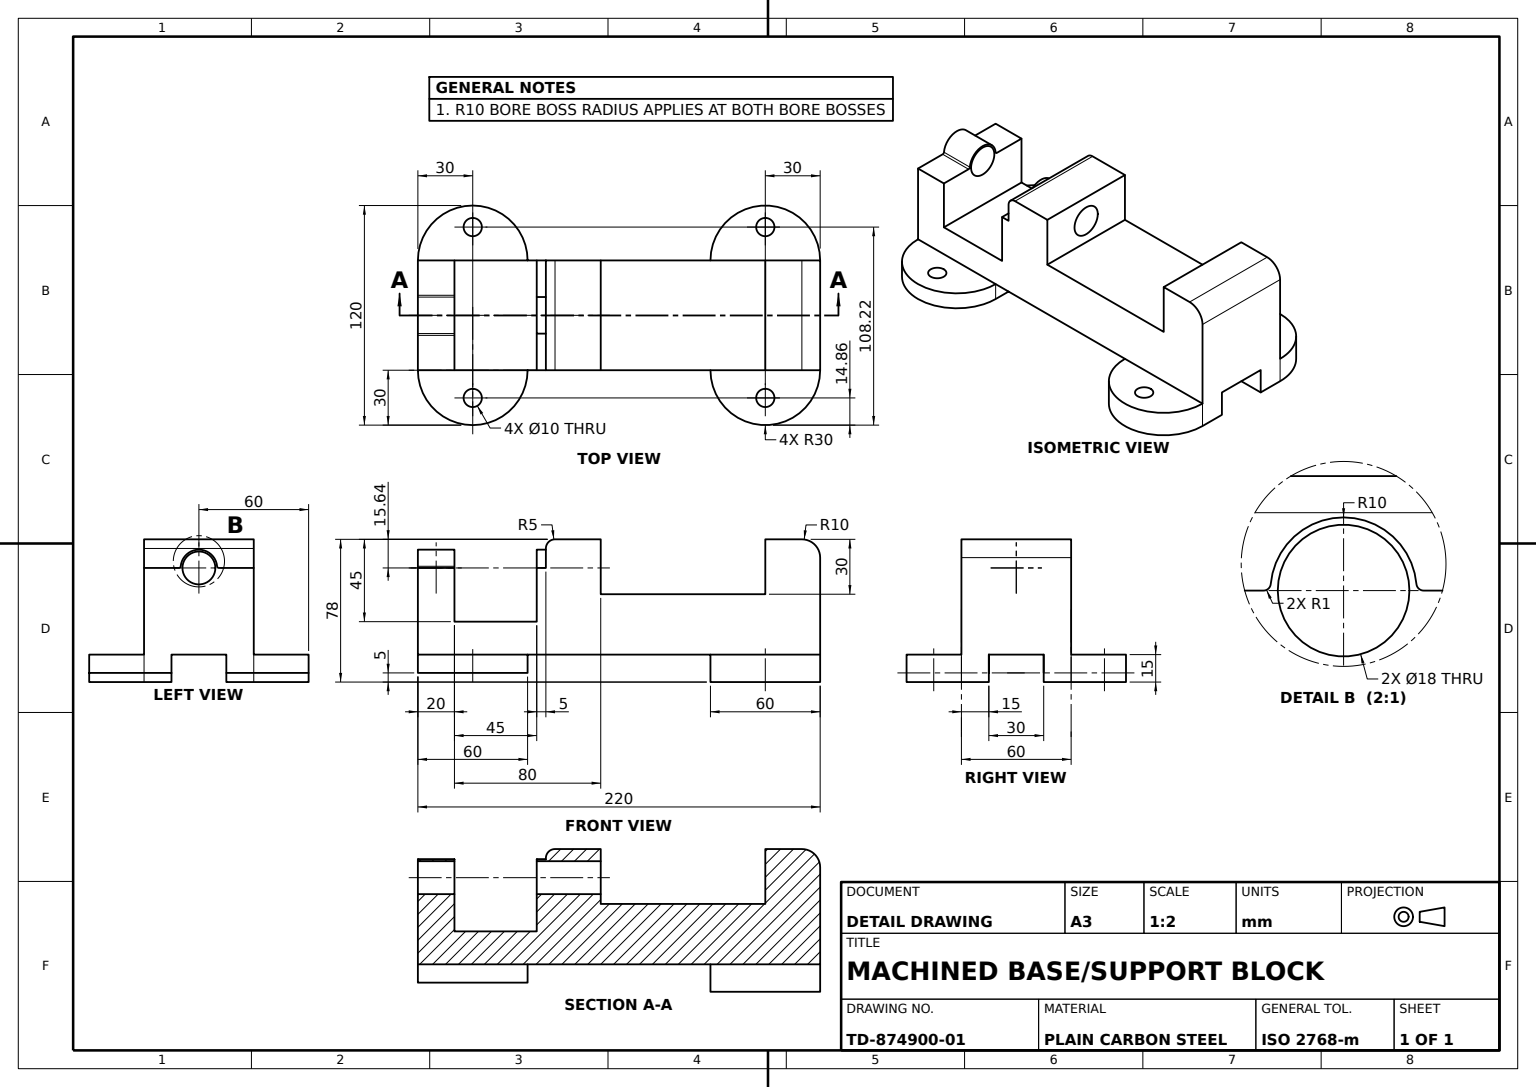
SolidWorks part; units mm, degrees
material "Plain Carbon Steel"
ref_plane "Front Plane" through (0, 0, 0) normal (0, 0, 1) x (1, 0, 0)
ref_plane "Top Plane" through (0, 0, 0) normal (0, 1, 0) x (1, 0, 0)
ref_plane "Right Plane" through (0, 0, 0) normal (1, 0, 0) x (0, 0, -1)
sketch "Base Plate Sketch" plane through (0, 0, 0) normal (0, 1, 0) x (1, 0, 0)
  line L0 (0, 0) -> (100, 0)
  line L1 (0, 0) -> (-100, 0)
  line L2 (100, 0) -> (100, 60)
  line L3 (100, 60) -> (-100, 60)
  line L4 (-100, 60) -> (-100, 0)
  dimension "D1" = 200
  dimension "D2" = 60
  dimension "D3" = 100
extrude "Base Plate" add sketch "Base Plate Sketch" along normal blind 15
sketch "Body Block Sketch" plane through (0, 15, 0) normal (0, 1, 0) x (1, 0, 0)
  line L0 (100, 0) -> (-100, 0)
  line L1 (-100, 0) -> (-100, 60)
  line L2 (-100, 60) -> (100, 60)
  line L3 (100, 60) -> (100, 0)
extrude "Body Block" add sketch "Body Block Sketch" along normal blind 48
sketch "Fixed Jaw Sketch" plane through (100, 0, 0) normal (1, 0, 0) x (0, 0, -1)
  line L0 (0, 0) -> (0, 63)
  line L1 (0, 63) -> (60, 63)
  line L2 (60, 63) -> (60, 0)
  line L3 (60, 0) -> (0, 0)
extrude "Fixed Jaw" add sketch "Fixed Jaw Sketch" along normal blind 20
sketch "Guide Channel Sketch" plane through (0, 63, 0) normal (0, 1, 0) x (1, 0, 0)
  line L0 (-100, 60) -> (90, 60)
  line L1 (120, 60) -> (120, 0) construction
  line L2 (90, 60) -> (0, 60)
  line L3 (90, 60) -> (30, 60)
  line L7 (30, 60) -> (30, 0)
  line L8 (-100, 0) -> (120, 0) construction
  line L9 (30, 0) -> (90, 0)
  line L10 (90, 60) -> (90, 0)
  line M9 (-100, 0) -> (120, 0)
  line M11 (120, 60) -> (-100, 60)
  dimension "D1" = 190
  dimension "D2" = 120
extrude "Guide Channel Cut" cut sketch "Guide Channel Sketch" against normal blind 30 contours L10 L7 M11 M9
sketch "Channel End Cut Sketch" plane through (0, 63, 0) normal (0, 1, 0) x (1, 0, 0)
  line L0 (30, 60) -> (0, 60)
  line L1 (30, 60) -> (-100, 60) construction
  line L2 (0, 60) -> (0, 0)
  line L3 (0, 0) -> (30, 0)
  line L4 (30, 0) -> (30, 60)
extrude "Channel End Cut" cut sketch "Channel End Cut Sketch" against normal blind 30
sketch "Jaw Slot Sketch" plane through (0, 63, 0) normal (0, 1, 0) x (1, 0, 0)
  line L1 (0, 60) -> (-100, 60) construction
  line L2 (-30, 60) -> (-30, 0)
  line L3 (-100, 0) -> (0, 0) construction
  line L5 (-30, 0) -> (-80, 0)
  line L6 (-80, 0) -> (-80, 60)
  line L7 (-80, 60) -> (-30, 60)
  line L8 (-80, 60) -> (-30, 60)
  line L9 (-80, 0) -> (-30, 0)
  line M3 (-100, 0) -> (0, 0)
  line M5 (0, 60) -> (-100, 60)
  dimension "D1" = 30
  dimension "D2" = 80
extrude "Jaw Slot Cut" cut sketch "Jaw Slot Sketch" against normal blind 45 contours L6 L2 M3 M5
sketch "Slot Rail Sketch" plane through (-30, 0, 0) normal (-1, 0, 0) x (0, 0, 1)
  line L0 (0, 47.3574) -> (0, 15)
  line L1 (0, 63) -> (0, 0) construction
  line L2 (-20, 47.3574) -> (0, 47.3574)
  line L3 (0, 15) -> (-60, 15)
  line L4 (-60, 63) -> (-60, 0) construction
  line L5 (-60, 15) -> (-60, 47.3574)
  line L6 (-60, 47.3574) -> (-40, 47.3574)
  line L7 (-60, 63) -> (0, 63) construction
  circle A0 centre (-30, 47.3574) radius 10
  line M4 (-60, 63) -> (-60, 18)
  line M5 (-60, 18) -> (0, 18)
  line M6 (0, 18) -> (0, 63)
  dimension "D1" = 20
  dimension "D2" = 15.6426
  dimension "D3" = 48
extrude "Slot Rail" add sketch "Slot Rail Sketch" along normal blind 5 contours A0 | A0 L6 L2 M4 M5 M6
sketch "Screw Bore Sketch" plane through (-35, 0, 0) normal (-1, 0, 0) x (0, 0, 1)
  circle A0 centre (-30, 47.3574) radius 9
  dimension "D1" = 18
extrude "Screw Bore" cut sketch "Screw Bore Sketch" against normal mid plane 158
sketch "Screw Pocket Sketch" plane through (-100, 0, 0) normal (-1, 0, 0) x (0, 0, 1)
  line L0 (-21, 47.3574) -> (0, 47.3574)
  line L2 (0, 0) -> (-60, 0)
  line L3 (-60, 47.3574) -> (-60, 63)
  line L4 (-60, 63) -> (0, 63)
  line L5 (-60, 63) -> (0, 63) construction
  line L6 (0, 63) -> (0, 0) construction
  line L7 (0, 63) -> (0, 47.3574)
  line L8 (-39, 47.3574) -> (-60, 47.3574)
  circle A0 centre (-30, 47.3574) radius 9 construction
  circle A1 centre (-30, 47.3574) radius 9
  circle M6 centre (-30, 47.3574) radius 9
  line M8 (0, 0) -> (0, 63)
  line M9 (0, 63) -> (-60, 63)
  line M10 (-60, 63) -> (-60, 0)
extrude "Screw Pocket Cut" cut sketch "Screw Pocket Sketch" against normal blind 40 contours L8 L0 M6 M8 M9 M10
sketch "Screw Boss Sketch" plane through (-100, 0, 0) normal (-1, 0, 0) x (0, 0, 1)
  circle A0 centre (-30, 47.3574) radius 9
  circle A1 centre (-30, 47.3574) radius 10
  dimension "D1" = 18
  dimension "D2" = 20
extrude "Screw Boss" add sketch "Screw Boss Sketch" against normal blind 20
fillet "Fixed Jaw Fillet R10" radius 10 1 edges at (120, 63, -30)
fillet "Jaw Slot Fillet R5" radius 5 1 edges at (-30, 63, -30)
fillet "Screw Boss Fillet R1 A" radius 1 1 edges at (-90, 47.3574, -20)
fillet "Screw Boss Fillet R1 B" radius 1 1 edges at (-90, 47.3574, -40)
sketch "Mounting Flange Sketch" plane through (0, 0, 0) normal (0, 0, 1) x (1, 0, 0)
  line L0 (-100, 0) -> (-100, -10)
  line L1 (-100, -10) -> (-40, -10)
  line L2 (-40, -10) -> (-40, 0)
  line L3 (-100, 0) -> (120, 0) construction
  line L4 (-40, 0) -> (-100, 0)
  line L5 (-80, 18) -> (-80, 47.3574) construction
  line L6 (-80, 18) -> (-35, 18) construction
  dimension "D1" = 40
  dimension "D2" = 28
extrude "Mounting Flange" add sketch "Mounting Flange Sketch" along normal blind 30 separate body
sketch "Flange Recess Sketch" plane through (0, 0, 0) normal (0, 1, 0) x (1, 0, 0)
  line L0 (-40, 0) -> (-100, 0) construction
  line L2 (-40, 0) -> (-40, -30)
  line L3 (-40, -30) -> (-100, -30)
  line L4 (-100, -30) -> (-100, 0)
  arc A0 (-100, 0) -> (-40, 0) centre (-70, 0) ccw
  line M3 (-100, 0) -> (-100, -30)
  line M4 (-100, -30) -> (-40, -30)
  line M5 (-40, -30) -> (-40, 0)
extrude "Flange Recess Cut" cut sketch "Flange Recess Sketch" against normal blind 15 contours A0 L3 M5 | A0 M3 M4
sketch "Mounting Lug Sketch" plane through (0, 0, 0) normal (0, 0, -1) x (-1, 0, 0)
  line L0 (40, 0) -> (100, 0)
  line L1 (100, 0) -> (100, -10)
  line L2 (100, -10) -> (40, -10)
  line L3 (40, -10) -> (40, 0)
extrude "Mounting Lug" add sketch "Mounting Lug Sketch" along normal blind 15
ref_plane "Plane1" through (0, 0, -30) normal (0, 0, 1) x (1, 0, 0)
mirror "Mounting Lug Mirror" about plane through (0, 0, -30) normal (0, 0, 1) of bodies 121
sketch "Rear Jaw Block Sketch" plane through (0, 0, 0) normal (0, 0, 1) x (1, 0, 0)
  line L0 (120, 0) -> (60, 0)
  line L1 (-40, 0) -> (120, 0) construction
  line L2 (60, 0) -> (60, -15)
  line L3 (60, -15) -> (120, -15)
  line L4 (120, -15) -> (120, 0)
  line L5 (120, 53) -> (120, 0) construction
  dimension "D1" = 60
  dimension "D2" = 15
extrude "Rear Jaw Block" add sketch "Rear Jaw Block Sketch" along normal blind 30 separate body
sketch "Rear Jaw Channel Sketch" plane through (0, 0, 0) normal (0, 1, 0) x (1, 0, 0)
  line L0 (60, 0) -> (120, 0)
  line L1 (120, 0) -> (120, -30)
  line L2 (120, -30) -> (60, -30)
  line L3 (60, -30) -> (60, 0)
  arc A0 (60, 0) -> (120, 0) centre (90, 0) ccw
  line M7 (60, 0) -> (60, -30)
  line M8 (60, -30) -> (120, -30)
extrude "Rear Jaw Channel Cut" cut sketch "Rear Jaw Channel Sketch" against normal blind 30 contours A0 M7 M8
sketch "Rear Jaw Notch Sketch" plane through (0, 0, 0) normal (0, 1, 0) x (1, 0, 0)
  line L0 (120, 0) -> (60, 0) construction
  line L1 (90, 0) -> (120, 0)
  line L2 (120, 0) -> (120, -30)
  line L3 (120, -30) -> (90, -30)
  line L4 (90, -30) -> (90, 0)
  arc A0 (60, 0) -> (120, 0) centre (90, 0) ccw
  line M4 (90, -30) -> (120, -30)
  line M5 (120, -30) -> (120, 0)
extrude "Rear Jaw Notch Cut" cut sketch "Rear Jaw Notch Sketch" against normal blind 30 contours A0 M4 M5
sketch "Rear Lug Sketch" plane through (0, 0, 0) normal (0, 0, -1) x (-1, 0, 0)
  line L0 (-120, 0) -> (-120, -15)
  line L1 (-120, -15) -> (-60, -15)
  line L2 (-60, -15) -> (-60, 0)
  line L3 (-60, 0) -> (-120, 0)
extrude "Rear Lug" add sketch "Rear Lug Sketch" along normal blind 15
mirror "Rear Lug Mirror" about plane through (0, 0, -30) normal (0, 0, 1) of bodies 132
sketch "Lug Clearance Cut Sketch" plane through (0, 0, 0) normal (0, 1, 0) x (1, 0, 0)
  line L0 (-40, 0) -> (-100, 0) construction
  circle A0 centre (-70, -15.1387) radius 5
  circle A1 centre (90, -15.1387) radius 5
  circle A2 centre (-70, 78.2236) radius 5
  circle A3 centre (90, 78.2236) radius 5
  dimension "D1" = 10
  dimension "D2" = 30
  dimension "D3" = 190
  dimension "D4" = 78.2236
  dimension "D5" = 15.1387
extrude "Lug Clearance Cut" cut sketch "Lug Clearance Cut Sketch" against normal blind 15
